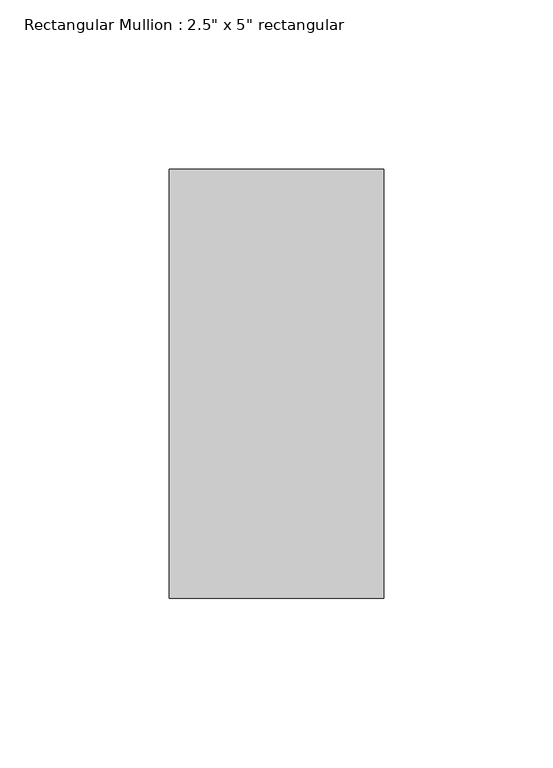
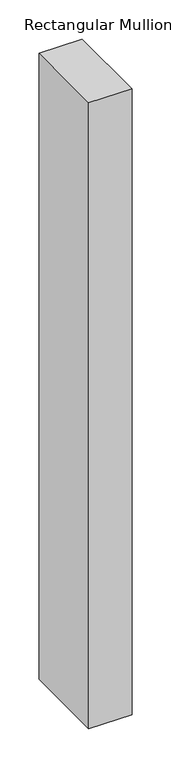
"""IFC4 building model written with IfcOpenShell, lengths in millimetres: member geometry."""

from ifc_helpers import new_model, si_unit, frame, origin, place, context, project, spatial, polyline, outline, extrude, source, transform, mapped, element, save


def member_4aea75b7(model_context):
    return source(origin(), model_context, "Body", "SweptSolid", [
        extrude(outline(polyline([(31.75, 63.5), (31.75, -63.5), (-31.75, -63.5), (-31.75, 63.5), (31.75, 63.5)])), frame((0.0, 0.0, -974.5210507), z_axis=(0.0, 0.0, 1.0), x_axis=(1.0, 0.0, 0.0)), (0.0, 0.0, 1.0), 974.5210507),
    ])


if __name__ == "__main__":
    model = new_model("IFC4")
    model_context = context("Model", 3, world=origin())
    ifc_project = project(units=[si_unit("LENGTHUNIT", "METRE", prefix="MILLI")], contexts=[model_context])
    site = spatial("IfcSite", under=ifc_project)
    building = spatial("IfcBuilding", under=site)
    placement = place(None, origin())
    member_shape = member_4aea75b7(model_context)
    element("IfcMember", 1, ObjectType="Rectangular Mullion : 2.5\" x 5\" rectangular", at=placement, inside=building, context=model_context, shape_type="MappedRepresentation", body=[
        mapped(member_shape, transform((0.0, 0.0, 0.0), x_axis=(1.0, 0.0, 0.0), y_axis=(0.0, 1.0, 0.0), z_axis=(0.0, 0.0, 1.0))),
    ])
    save(model, "model.ifc")

# Revit data of these elements
# Type "Rectangular Mullion : 2.5\" x 5\" rectangular"
#   built-in parameter 1007304 = 0.416667 (stored number, unit not read)
#   built-in parameter 1007301 = 0.104167 (stored number, unit not read)
#   built-in parameter 1007300 = 0.104167 (stored number, unit not read)
# Element 1 (IfcMember, "Rectangular Mullion : 2.5\" x 5\" rectangular")
#   Materials on its faces: "BLACK COLOUR"
# Materials
#   "BLACK COLOUR": class "Generic", colour RGB 120 120 120, transparency 0, Cost = 0
